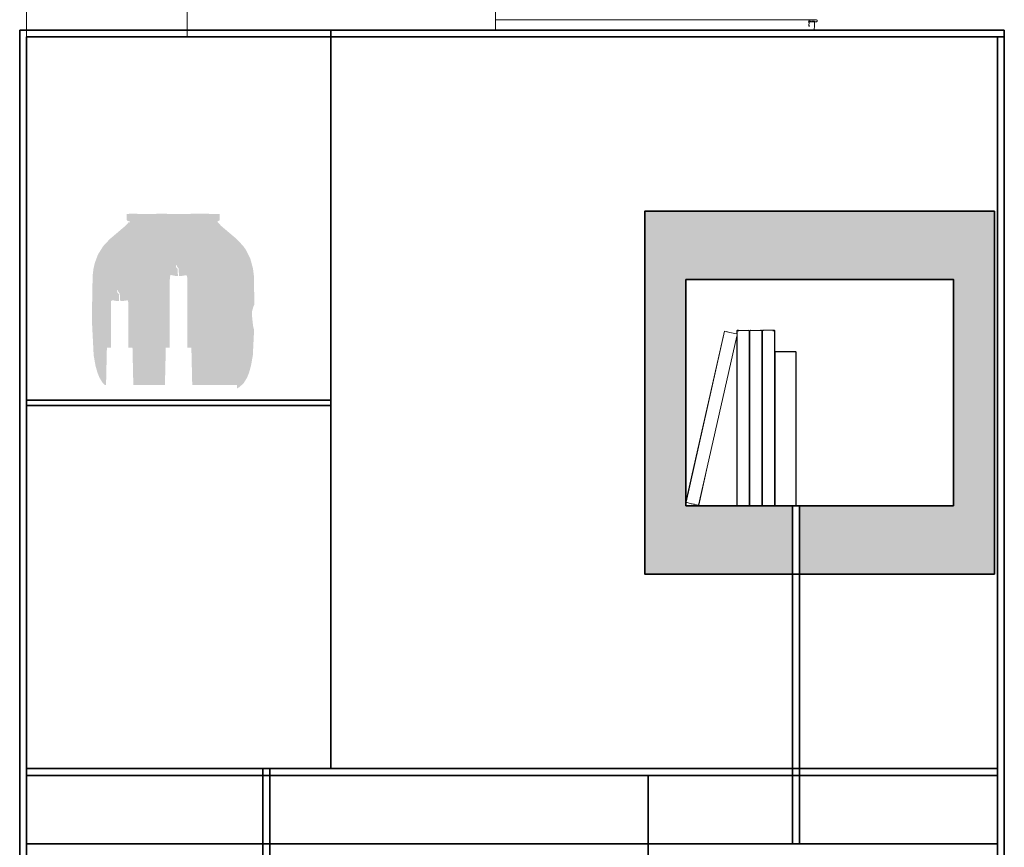
# Model space of a CAD drawing. Units: millimetres. Extents: x 2322 to 2394, y 1600 to 1790.
# Tile 4 of 5: x 2322 to 2394, y 1696 to 1757. Entities that reach past the tile are written whole.
import ezdxf

# ---------------------------------------------------------------- set-up
doc = ezdxf.new("R2010")
doc.units = ezdxf.units.MM
for name, color, linetype, lineweight in [('A-FURN', 7, 'Continuous', 35), ('A-FURN-ACCS', 8, 'Continuous', 18), ('A-FURN-PATT', 18, 'Continuous', 13)]:
    doc.layers.add(name, color=color, linetype=linetype, lineweight=lineweight)

msp = doc.modelspace()

# ---------------------------------------------------------------- hatches: boundary and pattern name
at = {"layer": 'A-FURN-PATT'}
h = msp.add_hatch(color=256, dxfattribs=at)
h.dxf.hatch_style = 1
h.paths.add_polyline_path([(2392.874, 1742.691), (2367.299, 1742.691), (2367.299, 1716.15), (2378.094, 1716.15), (2378.094, 1721.15), (2376.822, 1721.15), (2370.299, 1721.15), (2370.299, 1737.691), (2389.874, 1737.691), (2389.874, 1721.15), (2378.594, 1721.15), (2378.594, 1716.15), (2392.874, 1716.15)])
h.paths.add_polyline_path([(2352.154, 1685.571), (2339.867, 1685.571), (2339.867, 1680.571), (2349.154, 1680.571), (2349.154, 1664.029), (2329.579, 1664.029), (2329.579, 1680.571), (2339.367, 1680.571), (2339.367, 1685.571), (2326.579, 1685.571), (2326.579, 1659.029), (2352.154, 1659.029)])
h.paths.add_polyline_path([(2390.882, 1635.073), (2365.307, 1635.073), (2365.307, 1608.531), (2390.882, 1608.531)])
h.paths.add_polyline_path([(2387.882, 1630.073), (2387.882, 1613.531), (2368.307, 1613.531), (2368.307, 1630.073)], flags=16)
h.paths.add_polyline_path([(2373.463, 1622.711), (2373.46, 1622.644), (2373.462, 1622.642)], flags=0)
h.paths.add_polyline_path([(2380.387, 1618.619), (2380.387, 1618.619), (2380.35, 1618.619)], flags=0)
h.paths.add_polyline_path([(2377.431, 1618.132), (2377.363, 1618.141), (2377.19, 1618.152), (2377.145, 1618.149), (2376.982, 1618.132)], flags=0)
h.paths.add_polyline_path([(2376.126, 1618.152), (2375.767, 1618.152), (2375.734, 1618.152), (2375.734, 1618.152), (2375.028, 1618.152), (2375.028, 1618.198), (2374.578, 1618.295), (2374.235, 1618.449), (2373.926, 1618.69), (2373.709, 1619.163), (2373.66, 1619.336), (2373.672, 1619.402), (2373.73, 1620.54), (2373.702, 1622.038), (2373.678, 1622.131), (2373.705, 1621.917), (2373.73, 1620.54), (2373.667, 1619.311), (2373.709, 1619.163), (2373.87, 1618.812), (2373.949, 1618.699), (2374.037, 1618.604), (2374.187, 1618.486), (2374.3, 1618.42), (2374.485, 1618.337), (2374.688, 1618.272), (2374.979, 1618.209), (2375.028, 1618.203), (2375.028, 1618.372), (2375.028, 1618.619), (2377.125, 1618.619), (2377.165, 1620.356), (2377.172, 1620.356), (2377.172, 1620.357), (2377.341, 1620.357), (2377.354, 1620.357), (2377.354, 1623.532), (2377.38, 1623.766), (2377.629, 1623.72), (2377.726, 1623.72), (2377.722, 1623.891), (2377.719, 1624.041), (2377.644, 1624.123), (2377.631, 1624.228), (2377.644, 1624.211), (2377.677, 1624.213), (2377.688, 1624.153), (2377.757, 1624.059), (2377.78, 1623.72), (2377.883, 1623.72), (2378.152, 1623.76), (2378.155, 1620.358), (2378.298, 1620.356), (2378.301, 1620.356), (2378.362, 1620.357), (2378.402, 1618.619), (2377.354, 1618.619), (2377.125, 1618.619), (2375.028, 1618.619), (2375.028, 1618.372), (2375.028, 1618.177), (2375.049, 1618.152), (2375.734, 1618.152), (2375.756, 1618.153), (2375.767, 1618.152), (2376.126, 1618.152), (2376.144, 1618.154), (2376.168, 1618.151)], flags=0)
h.paths.add_polyline_path([(2380.5, 1618.343), (2380.401, 1618.342), (2380.5, 1618.342)], flags=0)
h.paths.add_polyline_path([(2378.836, 1627.111), (2378.86, 1627.114), (2378.771, 1627.114), (2378.773, 1627.108)], flags=0)
h.paths.add_polyline_path([(2378.972, 1627.091), (2379.09, 1626.957), (2378.972, 1626.879), (2378.964, 1626.862), (2378.975, 1626.787), (2379.128, 1626.434), (2379.25, 1626.246), (2379.42, 1626.03), (2379.646, 1625.791), (2380.15, 1625.354), (2380.519, 1624.956), (2380.743, 1624.553), (2380.884, 1624.119), (2380.94, 1623.673), (2380.977, 1621.652), (2380.892, 1619.98), (2380.807, 1619.502), (2380.712, 1619.163), (2380.621, 1618.942), (2380.422, 1618.619), (2380.413, 1618.619), (2380.386, 1618.619), (2380.474, 1618.703), (2380.621, 1618.942), (2380.712, 1619.163), (2380.807, 1619.502), (2380.892, 1619.98), (2380.977, 1621.652), (2380.94, 1623.673), (2380.9, 1623.987), (2380.843, 1624.244), (2380.778, 1624.446), (2380.693, 1624.644), (2380.585, 1624.839), (2380.452, 1625.029), (2380.15, 1625.354), (2379.646, 1625.791), (2379.324, 1626.132), (2379.128, 1626.434), (2378.92, 1626.915), (2378.841, 1626.975), (2378.869, 1626.811), (2379.027, 1626.915), (2379.041, 1626.939), (2379.037, 1626.997), (2379.02, 1627.036), (2378.879, 1627.196), (2378.841, 1627.151)], flags=0)
h.paths.add_polyline_path([(2375.501, 1627.114), (2375.642, 1627.103), (2375.561, 1626.855), (2375.555, 1626.827), (2375.48, 1626.868), (2375.292, 1626.434), (2375.097, 1626.132), (2374.775, 1625.791), (2374.271, 1625.354), (2374.13, 1625.216), (2373.969, 1625.029), (2373.836, 1624.839), (2373.728, 1624.644), (2373.643, 1624.446), (2373.537, 1624.119), (2373.52, 1623.987), (2373.601, 1624.348), (2373.773, 1624.748), (2374.034, 1625.122), (2374.271, 1625.354), (2374.775, 1625.791), (2375.001, 1626.03), (2375.171, 1626.246), (2375.292, 1626.434), (2375.445, 1626.787), (2375.447, 1626.797), (2375.334, 1627.042)], flags=0)
h.paths.add_polyline_path([(2375.398, 1627.114), (2375.384, 1626.997), (2375.411, 1627.054), (2375.531, 1627.169), (2375.597, 1627.114)], flags=0)
h.paths.add_polyline_path([(2377.985, 1623.628), (2377.785, 1623.645), (2377.786, 1623.634), (2377.764, 1623.634), (2377.729, 1623.636), (2377.728, 1623.656), (2377.701, 1623.664), (2377.421, 1623.752), (2377.412, 1623.748), (2377.629, 1623.72), (2377.78, 1623.72), (2377.783, 1623.68)], flags=0)
h.paths.add_polyline_path([(2377.348, 1620.357), (2377.335, 1620.357), (2377.327, 1620.356), (2377.354, 1620.356)], flags=0)
h.paths.add_polyline_path([(2377.834, 1620.357), (2377.854, 1620.356), (2377.911, 1620.356), (2377.923, 1620.357)], flags=0)
h.paths.add_polyline_path([(2378.155, 1620.356), (2378.155, 1620.356), (2378.014, 1620.356), (2378.002, 1620.357), (2377.96, 1620.356), (2377.956, 1620.356), (2377.923, 1620.357), (2378.111, 1620.357), (2378.119, 1620.356), (2378.144, 1620.356), (2378.163, 1620.357), (2378.163, 1620.357), (2378.157, 1620.357), (2378.149, 1620.356)], flags=0)
h.paths.add_polyline_path([(2377.609, 1620.357), (2377.623, 1620.356), (2377.653, 1620.357), (2377.738, 1620.356), (2377.743, 1620.357)], flags=0)
h.paths.add_polyline_path([(2380.479, 1618.152), (2380.406, 1618.152), (2380.313, 1618.151), (2380.107, 1618.152), (2380.104, 1618.152), (2380.108, 1618.151), (2379.961, 1618.152), (2379.793, 1618.152), (2377.32, 1618.152), (2377.3, 1618.149), (2377.253, 1618.152), (2379.793, 1618.152), (2380.01, 1618.153), (2380.21, 1618.152), (2380.229, 1618.152), (2380.231, 1618.152), (2380.394, 1618.152), (2380.48, 1618.152)], flags=0)
h = msp.add_hatch(color=256, dxfattribs=at)
h.dxf.hatch_style = 1
h.paths.add_polyline_path([(2332.999, 1738.736), (2333.07, 1738.74), (2333.086, 1738.645), (2333.198, 1738.496), (2333.234, 1737.954), (2333.398, 1737.954), (2333.785, 1738.013), (2333.827, 1737.85), (2333.831, 1732.707), (2333.857, 1732.707), (2333.873, 1732.707), (2333.989, 1732.707), (2333.994, 1732.707), (2334.135, 1732.707), (2334.198, 1729.992), (2337.241, 1729.992), (2337.298, 1729.991), (2337.317, 1729.991), (2337.475, 1729.993), (2337.475, 1729.726), (2337.671, 1729.848), (2337.964, 1730.127), (2338.2, 1730.51), (2338.344, 1730.86), (2338.495, 1731.396), (2338.628, 1732.151), (2338.721, 1733.987), (2338.642, 1734.328), (2338.558, 1735.144), (2338.575, 1735.376), (2338.671, 1735.726), (2338.743, 1735.863), (2338.704, 1737.987), (2338.642, 1738.485), (2338.448, 1739.21), (2338.143, 1739.831), (2337.933, 1740.132), (2337.456, 1740.645), (2336.31, 1741.616), (2336.022, 1741.94), (2336.183, 1742.002), (2336.212, 1742.049), (2336.212, 1742.467), (2336.13, 1742.495), (2335.712, 1742.495), (2335.163, 1742.497), (2334.435, 1742.497), (2333.692, 1742.495), (2332.796, 1742.495), (2331.964, 1742.497), (2331.952, 1742.497), (2331.142, 1742.495), (2330.425, 1742.495), (2329.946, 1742.497), (2329.586, 1742.497), (2329.426, 1742.483), (2329.415, 1742.478), (2329.4, 1742.447), (2329.407, 1742.049), (2329.432, 1742.006), (2329.646, 1741.923), (2329.625, 1741.887), (2329.578, 1741.831), (2329.562, 1741.89), (2329.309, 1741.616), (2328.163, 1740.645), (2327.686, 1740.132), (2327.305, 1739.523), (2327.068, 1738.891), (2326.977, 1738.485), (2326.915, 1737.987), (2326.856, 1734.794), (2326.99, 1732.151), (2327.124, 1731.396), (2327.275, 1730.86), (2327.419, 1730.51), (2327.654, 1730.127), (2327.797, 1729.992), (2327.895, 1729.992), (2327.957, 1732.707), (2328.08, 1732.707), (2328.256, 1732.707), (2328.263, 1736.124), (2328.376, 1736.177), (2328.691, 1736.119), (2328.847, 1736.119), (2328.84, 1736.391), (2328.835, 1736.629), (2328.716, 1736.76), (2328.699, 1736.899), (2328.769, 1736.903), (2328.785, 1736.807), (2328.896, 1736.659), (2328.933, 1736.119), (2329.096, 1736.118), (2329.482, 1736.177), (2329.525, 1736.014), (2329.531, 1732.707), (2329.582, 1732.707), (2329.621, 1732.707), (2329.727, 1732.707), (2329.828, 1732.707), (2329.89, 1729.992), (2332.202, 1729.992), (2332.265, 1732.707), (2332.388, 1732.707), (2332.554, 1732.708), (2332.554, 1737.655), (2332.596, 1738.029), (2332.992, 1737.953), (2333.148, 1737.953), (2333.141, 1738.228), (2333.136, 1738.466), (2333.017, 1738.597)])

# ---------------------------------------------------------------- linework, layer by layer
at = {"layer": 'A-FURN'}
for p, q in [((2321.58, 1599.925), (2321.58, 1755.925)), ((2321.58, 1755.925), (2393.58, 1755.925)), ((2322.08, 1755.425), (2322.08, 1701.937)), ((2322.08, 1600.425), (2322.08, 1755.425)), ((2322.08, 1755.425), (2393.58, 1755.425)), ((2322.08, 1755.425), (2333.831, 1755.425)), ((2344.339, 1755.925), (2344.339, 1701.937)), ((2393.08, 1755.425), (2393.08, 1600.425)), ((2393.58, 1755.925), (2393.58, 1599.925)), ((2392.874, 1742.691), (2392.874, 1716.15)), ((2322.08, 1728.881), (2344.339, 1728.881)), ((2322.08, 1728.481), (2344.339, 1728.481)), ((2378.094, 1696.437), (2378.094, 1721.15)), ((2378.594, 1696.437), (2378.594, 1721.15)), ((2322.08, 1701.937), (2393.08, 1701.937)), ((2322.08, 1701.437), (2393.08, 1701.437)), ((2339.367, 1680.571), (2339.367, 1701.937)), ((2339.867, 1680.571), (2339.867, 1701.937)), ((2367.535, 1701.437), (2367.535, 1648.381)), ((2322.08, 1696.437), (2393.08, 1696.437))]:
    msp.add_line(p, q, dxfattribs=at)
msp.add_lwpolyline([(2392.874, 1716.15), (2367.299, 1716.15), (2367.299, 1742.691), (2392.874, 1742.691)], dxfattribs=at)
msp.add_lwpolyline([(2389.874, 1721.15), (2370.299, 1721.15), (2370.299, 1737.691), (2389.874, 1737.691)], close=True, dxfattribs=at)
at = {"layer": 'A-FURN-ACCS'}
for p, q in [((2322.08, 1755.425), (2322.08, 1767.037)), ((2333.831, 1755.425), (2333.831, 1767.037)), ((2356.381, 1762.551), (2356.381, 1755.925)), ((2356.381, 1756.684), (2379.258, 1756.684)), ((2379.263, 1756.257), (2379.251, 1756.257)), ((2379.266, 1756.601), (2379.252, 1756.601)), ((2379.278, 1756.569), (2379.252, 1756.569)), ((2379.259, 1756.531), (2379.252, 1756.531)), ((2379.266, 1756.491), (2379.252, 1756.491)), ((2379.276, 1756.669), (2379.258, 1756.684)), ((2379.258, 1756.684), (2379.841, 1756.684)), ((2379.262, 1756.533), (2379.259, 1756.531)), ((2379.288, 1756.581), (2379.266, 1756.601)), ((2379.302, 1756.524), (2379.266, 1756.491)), ((2379.299, 1756.649), (2379.276, 1756.669)), ((2379.276, 1756.669), (2379.301, 1756.651)), ((2379.298, 1756.257), (2379.302, 1756.485)), ((2379.301, 1756.17), (2379.298, 1756.257)), ((2379.342, 1756.257), (2379.298, 1756.257)), ((2379.304, 1756.567), (2379.299, 1756.571)), ((2379.303, 1756.571), (2379.299, 1756.571)), ((2379.304, 1756.564), (2379.299, 1756.561)), ((2379.299, 1756.537), (2379.304, 1756.564)), ((2379.302, 1756.532), (2379.299, 1756.537)), ((2379.302, 1756.537), (2379.299, 1756.537)), ((2379.304, 1756.645), (2379.301, 1756.651)), ((2379.301, 1756.648), (2379.301, 1756.651)), ((2379.304, 1756.645), (2379.301, 1756.648)), ((2379.313, 1756.534), (2379.302, 1756.537)), ((2379.302, 1756.524), (2379.302, 1756.532)), ((2379.312, 1756.532), (2379.302, 1756.524)), ((2379.302, 1756.485), (2379.302, 1756.524)), ((2379.303, 1756.571), (2379.307, 1756.612)), ((2379.31, 1756.573), (2379.303, 1756.571)), ((2379.303, 1756.571), (2379.304, 1756.567)), ((2379.307, 1756.612), (2379.304, 1756.645)), ((2379.312, 1756.559), (2379.304, 1756.567)), ((2379.304, 1756.564), (2379.304, 1756.567)), ((2379.31, 1756.573), (2379.307, 1756.612)), ((2379.32, 1756.578), (2379.31, 1756.573)), ((2379.318, 1756.571), (2379.31, 1756.573)), ((2379.312, 1756.559), (2379.31, 1756.573)), ((2379.312, 1756.532), (2379.313, 1756.534)), ((2379.313, 1756.534), (2379.314, 1756.545)), ((2379.397, 1756.537), (2379.313, 1756.534)), ((2379.314, 1756.545), (2379.317, 1756.567)), ((2379.317, 1756.567), (2379.318, 1756.571)), ((2379.318, 1756.571), (2379.32, 1756.578)), ((2379.348, 1756.57), (2379.318, 1756.571)), ((2379.435, 1756.571), (2379.348, 1756.57)), ((2379.691, 1756.537), (2379.397, 1756.537)), ((2379.489, 1756.571), (2379.493, 1756.57)), ((2379.691, 1756.571), (2379.493, 1756.57)), ((2379.689, 1756.257), (2379.687, 1755.925)), ((2379.691, 1756.537), (2379.689, 1756.257)), ((2379.691, 1756.571), (2379.691, 1756.537)), ((2379.691, 1756.537), (2379.841, 1756.537)), ((2379.841, 1756.684), (2379.887, 1756.643)), ((2379.887, 1756.578), (2379.841, 1756.537)), ((2379.887, 1756.643), (2379.887, 1756.578)), ((2370.299, 1721.435), (2373.122, 1733.917)), ((2373.124, 1733.917), (2370.307, 1721.425)), ((2373.122, 1733.917), (2373.124, 1733.917)), ((2373.124, 1733.917), (2373.233, 1733.902)), ((2373.509, 1733.83), (2373.233, 1733.902)), ((2373.509, 1733.83), (2373.285, 1733.88)), ((2373.991, 1733.721), (2373.509, 1733.83)), ((2374.031, 1733.966), (2374.017, 1733.923)), ((2374.017, 1733.923), (2374.017, 1733.724)), ((2374.031, 1733.931), (2374.031, 1733.966)), ((2374.031, 1733.966), (2374.041, 1733.966)), ((2374.041, 1733.966), (2374.044, 1733.968)), ((2374.041, 1733.966), (2374.041, 1733.713)), ((2374.044, 1733.968), (2374.066, 1733.98)), ((2374.044, 1733.968), (2374.079, 1733.973)), ((2374.057, 1733.966), (2374.044, 1733.968)), ((2374.083, 1733.971), (2374.057, 1733.966)), ((2374.094, 1733.966), (2374.057, 1733.966)), ((2374.122, 1733.98), (2374.066, 1733.98)), ((2374.079, 1733.973), (2374.066, 1733.98)), ((2374.079, 1733.973), (2374.08, 1733.973)), ((2374.08, 1733.973), (2374.122, 1733.98)), ((2374.083, 1733.971), (2374.08, 1733.973)), ((2374.084, 1733.972), (2374.083, 1733.971)), ((2374.122, 1733.98), (2374.084, 1733.972)), ((2374.093, 1733.966), (2374.084, 1733.972)), ((2374.094, 1733.966), (2374.093, 1733.966)), ((2374.095, 1733.923), (2374.094, 1733.966)), ((2374.097, 1733.966), (2374.094, 1733.966)), ((2374.095, 1733.966), (2374.094, 1733.966)), ((2374.095, 1733.923), (2374.095, 1733.966)), ((2374.097, 1733.966), (2374.095, 1733.966)), ((2374.097, 1733.966), (2374.122, 1733.98)), ((2374.119, 1733.967), (2374.097, 1733.966)), ((2374.122, 1733.98), (2374.119, 1733.967)), ((2374.119, 1733.967), (2374.121, 1733.925)), ((2374.119, 1733.967), (2374.119, 1733.925)), ((2374.122, 1733.967), (2374.119, 1733.967)), ((2374.144, 1733.967), (2374.122, 1733.98)), ((2374.122, 1733.98), (2374.122, 1733.967)), ((2374.122, 1733.967), (2374.124, 1733.925)), ((2374.144, 1733.967), (2374.122, 1733.967)), ((2374.147, 1733.966), (2374.144, 1733.967)), ((2374.839, 1733.979), (2374.147, 1733.966)), ((2374.147, 1733.966), (2374.148, 1733.926)), ((2374.818, 1733.962), (2374.818, 1733.966)), ((2374.841, 1733.98), (2374.839, 1733.979)), ((2374.842, 1733.979), (2374.839, 1733.979)), ((2374.84, 1733.964), (2374.84, 1733.966)), ((2374.841, 1733.98), (2374.842, 1733.979)), ((2374.842, 1733.979), (2374.897, 1733.98)), ((2374.843, 1733.964), (2374.843, 1733.966)), ((2374.877, 1733.966), (2374.905, 1733.966)), ((2374.903, 1733.97), (2374.886, 1733.972)), ((2374.903, 1733.97), (2374.897, 1733.98)), ((2374.927, 1733.966), (2374.903, 1733.97)), ((2374.905, 1733.966), (2374.903, 1733.97)), ((2374.905, 1733.966), (2374.927, 1733.966)), ((2374.931, 1733.923), (2374.905, 1733.966)), ((2374.931, 1733.966), (2374.927, 1733.966)), ((2374.927, 1733.966), (2374.946, 1733.923)), ((2374.928, 1721.153), (2374.931, 1733.923)), ((2374.946, 1733.923), (2374.931, 1733.966)), ((2374.946, 1733.923), (2374.931, 1721.159)), ((2374.946, 1733.923), (2374.964, 1733.966)), ((2374.946, 1721.193), (2374.946, 1733.923)), ((2374.964, 1721.15), (2374.946, 1733.923)), ((2374.96, 1721.15), (2374.946, 1733.923)), ((2374.961, 1733.923), (2374.966, 1733.931)), ((2374.969, 1721.15), (2374.961, 1733.923)), ((2374.993, 1733.97), (2374.964, 1733.966)), ((2374.966, 1733.931), (2374.964, 1733.931)), ((2374.966, 1733.931), (2374.986, 1733.966)), ((2374.993, 1733.97), (2374.986, 1733.966)), ((2375.006, 1733.98), (2374.993, 1733.97)), ((2375.012, 1733.974), (2374.993, 1733.97)), ((2375.006, 1733.98), (2375.012, 1733.974)), ((2375.049, 1733.979), (2375.006, 1733.98)), ((2375.022, 1733.975), (2375.012, 1733.974)), ((2375.012, 1733.974), (2375.02, 1733.966)), ((2375.02, 1733.966), (2375.024, 1733.966)), ((2375.024, 1733.966), (2375.035, 1733.971)), ((2375.024, 1733.966), (2375.048, 1733.966)), ((2375.048, 1733.966), (2375.048, 1733.967)), ((2375.054, 1733.966), (2375.048, 1733.966)), ((2375.049, 1733.979), (2375.051, 1733.98)), ((2375.051, 1733.98), (2375.052, 1733.979)), ((2375.758, 1733.966), (2375.052, 1733.979)), ((2375.758, 1733.966), (2375.767, 1733.98)), ((2375.772, 1733.966), (2375.758, 1733.966)), ((2375.767, 1733.98), (2375.83, 1733.98)), ((2375.772, 1733.968), (2375.772, 1733.966)), ((2375.806, 1733.966), (2375.772, 1733.966)), ((2375.835, 1733.966), (2375.798, 1733.974)), ((2375.835, 1733.966), (2375.83, 1733.98)), ((2375.84, 1733.96), (2375.835, 1733.966)), ((2375.86, 1733.923), (2375.84, 1733.96)), ((2375.874, 1733.923), (2375.84, 1733.96)), ((2375.859, 1723.736), (2375.874, 1733.923)), ((2375.874, 1733.923), (2375.859, 1721.193)), ((2375.859, 1723.736), (2375.86, 1733.923)), ((2375.874, 1721.193), (2375.89, 1733.923)), ((2375.89, 1733.923), (2375.889, 1733.966)), ((2375.889, 1733.966), (2375.892, 1733.966)), ((2375.89, 1733.923), (2375.892, 1733.966)), ((2375.89, 1733.923), (2375.891, 1732.191)), ((2375.925, 1733.98), (2375.892, 1733.966)), ((2375.892, 1733.966), (2375.893, 1733.966)), ((2375.934, 1733.973), (2375.893, 1733.966)), ((2375.925, 1733.98), (2376.742, 1733.98)), ((2375.953, 1733.966), (2375.977, 1733.966)), ((2375.977, 1733.966), (2375.977, 1733.964)), ((2375.981, 1733.964), (2375.98, 1733.966)), ((2375.999, 1733.966), (2376.005, 1733.966)), ((2376.005, 1733.962), (2376.005, 1733.966)), ((2376.686, 1733.966), (2376.683, 1733.926)), ((2376.701, 1733.966), (2376.696, 1733.925)), ((2376.701, 1733.966), (2376.699, 1733.925)), ((2376.701, 1733.925), (2376.701, 1733.966)), ((2376.725, 1733.923), (2376.725, 1733.966)), ((2376.728, 1733.923), (2376.729, 1733.966)), ((2376.773, 1733.968), (2376.742, 1733.98)), ((2376.755, 1733.971), (2376.757, 1733.969)), ((2376.757, 1733.969), (2376.773, 1733.968)), ((2376.773, 1733.968), (2376.763, 1733.966)), ((2376.779, 1733.966), (2376.773, 1733.968)), ((2376.779, 1733.966), (2376.78, 1721.15)), ((2376.784, 1733.966), (2376.779, 1733.966)), ((2376.789, 1733.966), (2376.784, 1733.966)), ((2376.784, 1733.966), (2376.789, 1733.956)), ((2376.803, 1733.923), (2376.789, 1733.966)), ((2376.789, 1733.966), (2376.789, 1733.956)), ((2376.789, 1733.956), (2376.789, 1733.931)), ((2376.789, 1733.956), (2376.803, 1733.923)), ((2376.803, 1721.193), (2376.803, 1733.923)), ((2374.016, 1733.549), (2371.856, 1723.973)), ((2374.01, 1733.727), (2373.991, 1733.721)), ((2373.991, 1733.721), (2374.041, 1733.71)), ((2374.01, 1733.727), (2374.017, 1733.724)), ((2374.016, 1733.549), (2374.041, 1733.661)), ((2374.016, 1733.549), (2374.017, 1721.193)), ((2374.041, 1733.713), (2374.017, 1733.724)), ((2374.017, 1733.724), (2374.017, 1733.719)), ((2374.041, 1733.661), (2374.04, 1721.15)), ((2374.05, 1733.708), (2374.041, 1733.713)), ((2374.041, 1733.713), (2374.041, 1733.71)), ((2374.05, 1733.708), (2374.041, 1733.71)), ((2374.041, 1733.668), (2374.05, 1733.708)), ((2374.041, 1733.668), (2374.041, 1733.661)), ((2376.803, 1721.193), (2376.815, 1732.374)), ((2376.815, 1732.411), (2376.818, 1732.411)), ((2376.815, 1732.374), (2376.818, 1732.411)), ((2376.815, 1732.374), (2376.815, 1732.411)), ((2376.815, 1732.374), (2376.817, 1731.818)), ((2376.851, 1732.423), (2376.818, 1732.411)), ((2376.857, 1732.411), (2376.818, 1732.411)), ((2376.851, 1732.423), (2376.862, 1732.411)), ((2378.267, 1732.423), (2376.851, 1732.423)), ((2376.883, 1732.411), (2376.851, 1732.423)), ((2376.862, 1732.411), (2376.857, 1732.411)), ((2376.865, 1732.411), (2376.862, 1732.411)), ((2376.862, 1732.411), (2376.863, 1732.411)), ((2376.863, 1732.411), (2376.865, 1732.411)), ((2376.883, 1732.411), (2376.865, 1732.411)), ((2376.883, 1732.411), (2376.895, 1732.411)), ((2376.895, 1732.411), (2376.898, 1732.411)), ((2376.898, 1732.411), (2378.249, 1732.411)), ((2378.249, 1732.411), (2378.267, 1732.423)), ((2378.269, 1732.42), (2378.249, 1732.411)), ((2378.249, 1732.411), (2378.269, 1732.411)), ((2378.267, 1732.423), (2378.269, 1732.423)), ((2378.269, 1732.42), (2378.269, 1732.423)), ((2378.304, 1732.423), (2378.269, 1732.423)), ((2378.299, 1732.418), (2378.269, 1732.423)), ((2378.269, 1732.411), (2378.269, 1732.42)), ((2378.271, 1732.411), (2378.269, 1732.42)), ((2378.277, 1732.411), (2378.269, 1732.42)), ((2378.271, 1732.411), (2378.269, 1732.411)), ((2378.271, 1732.411), (2378.277, 1732.411)), ((2378.293, 1732.411), (2378.277, 1732.411)), ((2378.293, 1732.411), (2378.299, 1732.418)), ((2378.293, 1732.411), (2378.328, 1732.413)), ((2378.299, 1732.418), (2378.304, 1732.423)), ((2378.328, 1732.413), (2378.299, 1732.418)), ((2378.328, 1732.413), (2378.304, 1732.423)), ((2378.333, 1732.411), (2378.328, 1732.413)), ((2378.333, 1721.15), (2378.333, 1732.411)), ((2378.337, 1732.411), (2378.333, 1732.411)), ((2378.34, 1732.411), (2378.337, 1732.411)), ((2378.337, 1732.411), (2378.34, 1732.403)), ((2378.351, 1732.374), (2378.34, 1732.411)), ((2378.34, 1732.411), (2378.34, 1732.403)), ((2378.34, 1732.403), (2378.34, 1732.381)), ((2378.34, 1732.403), (2378.351, 1732.374)), ((2378.351, 1721.184), (2378.351, 1732.374)), ((2375.891, 1732.191), (2375.874, 1721.193)), ((2375.891, 1732.191), (2375.898, 1721.15)), ((2376.817, 1731.818), (2376.815, 1729.764)), ((2376.815, 1729.764), (2376.803, 1721.193)), ((2376.814, 1721.157), (2376.815, 1729.764)), ((2376.815, 1729.764), (2376.822, 1721.15)), ((2371.23, 1721.196), (2371.856, 1723.973)), ((2371.856, 1723.973), (2371.232, 1721.196)), ((2375.859, 1721.193), (2375.859, 1723.736)), ((2370.299, 1721.435), (2370.303, 1721.405)), ((2370.303, 1721.405), (2370.307, 1721.425)), ((2370.303, 1721.405), (2370.304, 1721.405)), ((2370.307, 1721.425), (2370.304, 1721.405)), ((2370.399, 1721.383), (2370.304, 1721.405)), ((2370.399, 1721.383), (2370.69, 1721.308)), ((2370.69, 1721.308), (2370.767, 1721.301)), ((2371.215, 1721.19), (2370.69, 1721.308)), ((2370.911, 1721.268), (2370.767, 1721.301)), ((2370.911, 1721.268), (2370.914, 1721.267)), ((2371.215, 1721.19), (2371.179, 1721.206)), ((2371.215, 1721.19), (2371.216, 1721.199)), ((2371.215, 1721.19), (2371.23, 1721.196)), ((2371.232, 1721.196), (2371.23, 1721.196)), ((2374.017, 1721.193), (2374.031, 1721.15)), ((2374.031, 1721.159), (2374.017, 1721.193)), ((2374.031, 1721.15), (2374.031, 1721.159)), ((2374.036, 1721.15), (2374.031, 1721.159)), ((2374.031, 1721.15), (2374.036, 1721.15)), ((2374.04, 1721.15), (2374.036, 1721.15)), ((2374.04, 1721.15), (2374.928, 1721.15)), ((2374.931, 1721.159), (2374.928, 1721.153)), ((2374.928, 1721.15), (2374.928, 1721.153)), ((2374.928, 1721.15), (2374.931, 1721.15)), ((2374.931, 1721.15), (2374.946, 1721.193)), ((2374.946, 1721.193), (2374.931, 1721.159)), ((2374.931, 1721.159), (2374.931, 1721.15)), ((2374.96, 1721.15), (2374.931, 1721.15)), ((2374.964, 1721.15), (2374.96, 1721.15)), ((2374.964, 1721.15), (2374.969, 1721.15)), ((2375.851, 1721.15), (2374.969, 1721.15)), ((2375.856, 1721.173), (2375.851, 1721.15)), ((2375.856, 1721.15), (2375.851, 1721.15)), ((2375.859, 1721.193), (2375.856, 1721.173)), ((2375.856, 1721.15), (2375.856, 1721.173)), ((2375.86, 1721.15), (2375.856, 1721.15)), ((2375.859, 1721.193), (2375.86, 1721.15)), ((2375.889, 1721.15), (2375.86, 1721.15)), ((2375.874, 1721.193), (2375.889, 1721.15)), ((2375.889, 1721.159), (2375.874, 1721.193)), ((2375.889, 1721.15), (2375.889, 1721.159)), ((2375.893, 1721.15), (2375.889, 1721.159)), ((2375.889, 1721.15), (2375.893, 1721.15)), ((2375.898, 1721.15), (2375.893, 1721.15)), ((2375.898, 1721.15), (2376.78, 1721.15)), ((2376.784, 1721.15), (2376.78, 1721.15)), ((2376.789, 1721.159), (2376.784, 1721.15)), ((2376.784, 1721.15), (2376.789, 1721.15)), ((2376.789, 1721.15), (2376.803, 1721.193)), ((2376.803, 1721.193), (2376.789, 1721.159)), ((2376.789, 1721.185), (2376.789, 1721.159)), ((2376.789, 1721.159), (2376.789, 1721.15)), ((2376.814, 1721.15), (2376.789, 1721.15)), ((2376.803, 1721.184), (2376.803, 1721.193)), ((2376.803, 1721.184), (2376.814, 1721.15)), ((2376.814, 1721.157), (2376.803, 1721.184)), ((2376.814, 1721.15), (2376.814, 1721.157)), ((2376.817, 1721.15), (2376.814, 1721.157)), ((2376.817, 1721.15), (2376.814, 1721.15)), ((2376.822, 1721.15), (2376.817, 1721.15)), ((2378.333, 1721.15), (2376.822, 1721.15)), ((2378.337, 1721.15), (2378.333, 1721.15)), ((2378.34, 1721.156), (2378.337, 1721.15)), ((2378.341, 1721.15), (2378.337, 1721.15)), ((2378.351, 1721.184), (2378.34, 1721.156)), ((2378.34, 1721.156), (2378.341, 1721.15)), ((2378.341, 1721.15), (2378.351, 1721.184))]:
    msp.add_line(p, q, dxfattribs=at)

doc.saveas('drawing.dxf')
